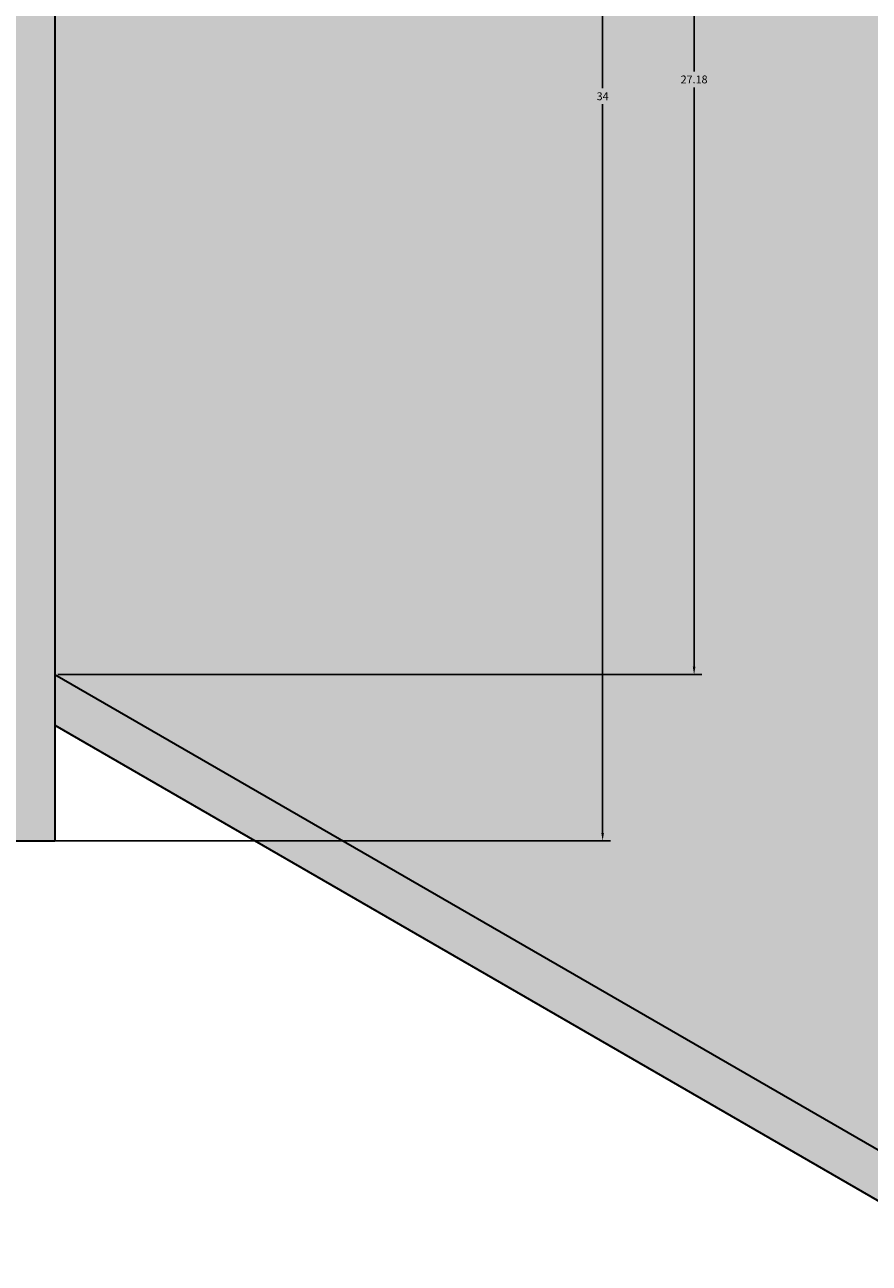
# Model space of a CAD drawing. Units: inches. Extents: x -1 to 292, y -3 to 199.
# Tile 7 of 52: x 23 to 43, y 45 to 73. Entities that reach past the tile are written whole.
import ezdxf

# ---------------------------------------------------------------- set-up
doc = ezdxf.new("R2010")
doc.units = ezdxf.units.IN
doc.header["$MEASUREMENT"] = 0
for name, color, linetype, lineweight in [('M-DIMS', 2, 'Continuous', 18), ('M-EQPM', 7, 'Continuous', 35), ('M-PATT', 8, 'Continuous', 13)]:
    doc.layers.add(name, color=color, linetype=linetype, lineweight=lineweight)
doc.styles.get("Standard").update_dxf_attribs({"font": 'arial.ttf'})
doc.dimstyles.get("Standard").update_dxf_attribs({"dimtxt": 0.18, "dimasz": 0.18, "dimexe": 0.18, "dimexo": 0.0625, "dimgap": 0.09, "dimtad": 0, "dimtih": 1, "dimtoh": 1, "dimdec": 4, "dimzin": 0, "dimdsep": 46, "dimtxsty": 'Standard', "dimcen": 0.09, "dimadec": 0, "dimazin": 0, "dimtfac": 1, "dimtdec": 4, "dimtofl": 0, "dimtmove": 0, "dimatfit": 3, "dimfxl": 1, "dimtolj": 1, "dimtzin": 0, "dimarcsym": 0})

# ---------------------------------------------------------------- blocks, each defined once
blk = doc.blocks.new('DUCT-FLANGE')
for p in [(2.089, 34), (0, 0)]:
    blk.add_line(p, (2.089, 0))
blk = doc.blocks.new('*D7')
at = {"layer": 'Defpoints', "color": 0, "transparency": 16777216}
for p in [(21.861, 54.582), (205.115, 54.582), (21.861, 39.982)]:
    blk.add_point(p, dxfattribs=at)
at = {"layer": 'M-DIMS', "color": 0, "lineweight": -2, "transparency": 16777216}
for p, q in [((21.861, 54.52), (21.861, 39.802)), ((205.115, 54.52), (205.115, 39.802)), ((22.041, 39.982), (113.033, 39.982)), ((204.935, 39.982), (113.944, 39.982))]:
    blk.add_line(p, q, dxfattribs=at)
at = {"layer": 'M-DIMS', "color": 0, "transparency": 16777216}
for points in [[(22.041, 40.012), (22.041, 39.952), (21.861, 39.982)], [(204.935, 40.012), (204.935, 39.952), (205.115, 39.982)]]:
    blk.add_solid(points, dxfattribs=at)
at = {"layer": 'M-DIMS', "color": 0, "transparency": 16777216, "insert": (113.488, 39.982), "char_height": 0.18, "attachment_point": 5}
blk.add_mtext('\\A1;183.25', dxfattribs=at)
blk = doc.blocks.new('*D8')
at = {"layer": 'Defpoints', "color": 0, "transparency": 16777216}
for p in [(-0.662, 126.765), (111.488, 126.765), (69.013, 25.514)]:
    blk.add_point(p, dxfattribs=at)
at = {"layer": 'M-DIMS', "color": 0, "lineweight": -2, "transparency": 16777216}
for p, q in [((111.426, 126.765), (-0.842, 126.765)), ((-0.662, 126.585), (-0.662, 76.321)), ((-0.662, 25.694), (-0.662, 75.958)), ((68.951, 25.514), (-0.842, 25.514))]:
    blk.add_line(p, q, dxfattribs=at)
at = {"layer": 'M-DIMS', "color": 0, "transparency": 16777216}
for points in [[(-0.692, 126.585), (-0.632, 126.585), (-0.662, 126.765)], [(-0.692, 25.694), (-0.632, 25.694), (-0.662, 25.514)]]:
    blk.add_solid(points, dxfattribs=at)
at = {"layer": 'M-DIMS', "color": 0, "transparency": 16777216, "insert": (-0.662, 76.14), "char_height": 0.18, "attachment_point": 5}
blk.add_mtext('\\A1;101.25', dxfattribs=at)
blk = doc.blocks.new('*D14')
at = {"layer": 'Defpoints', "color": 0, "transparency": 16777216}
for p in [(21.861, 88.582), (21.861, 54.582), (36.461, 54.582)]:
    blk.add_point(p, dxfattribs=at)
at = {"layer": 'M-DIMS', "color": 0, "lineweight": -2, "transparency": 16777216}
for p, q in [((21.924, 88.582), (36.641, 88.582)), ((36.461, 88.402), (36.461, 71.764)), ((36.461, 54.762), (36.461, 71.4)), ((21.924, 54.582), (36.641, 54.582))]:
    blk.add_line(p, q, dxfattribs=at)
at = {"layer": 'M-DIMS', "color": 0, "transparency": 16777216}
for points in [[(36.431, 88.402), (36.491, 88.402), (36.461, 88.582)], [(36.431, 54.762), (36.491, 54.762), (36.461, 54.582)]]:
    blk.add_solid(points, dxfattribs=at)
at = {"layer": 'M-DIMS', "color": 0, "transparency": 16777216, "insert": (36.461, 71.582), "char_height": 0.18, "attachment_point": 5}
blk.add_mtext('\\A1;34', dxfattribs=at)
blk = doc.blocks.new('*D17')
at = {"layer": 'Defpoints', "color": 0, "transparency": 16777216}
for p in [(23.95, 85.555), (23.95, 58.376), (38.55, 58.376)]:
    blk.add_point(p, dxfattribs=at)
at = {"layer": 'M-DIMS', "color": 0, "lineweight": -2, "transparency": 16777216}
for p, q in [((24.013, 85.555), (38.73, 85.555)), ((38.55, 85.375), (38.55, 72.147)), ((38.55, 58.556), (38.55, 71.784)), ((24.013, 58.376), (38.73, 58.376))]:
    blk.add_line(p, q, dxfattribs=at)
at = {"layer": 'M-DIMS', "color": 0, "transparency": 16777216}
for points in [[(38.52, 85.375), (38.58, 85.375), (38.55, 85.555)], [(38.52, 58.556), (38.58, 58.556), (38.55, 58.376)]]:
    blk.add_solid(points, dxfattribs=at)
at = {"layer": 'M-DIMS', "color": 0, "transparency": 16777216, "insert": (38.55, 71.966), "char_height": 0.18, "attachment_point": 5}
blk.add_mtext('\\A1;27.18', dxfattribs=at)
blk = doc.blocks.new('*D23')
at = {"layer": 'Defpoints', "color": 0, "transparency": 16777216}
for p in [(21.861, 54.582), (64.679, 51.267), (64.679, -2.71)]:
    blk.add_point(p, dxfattribs=at)
at = {"layer": 'M-DIMS', "color": 0, "lineweight": -2, "transparency": 16777216}
for p, q in [((21.861, 54.52), (21.861, -2.89)), ((64.679, 51.205), (64.679, -2.89)), ((22.041, -2.71), (42.874, -2.71)), ((64.499, -2.71), (43.666, -2.71))]:
    blk.add_line(p, q, dxfattribs=at)
at = {"layer": 'M-DIMS', "color": 0, "transparency": 16777216}
for points in [[(22.041, -2.68), (22.041, -2.74), (21.861, -2.71)], [(64.499, -2.68), (64.499, -2.74), (64.679, -2.71)]]:
    blk.add_solid(points, dxfattribs=at)
at = {"layer": 'M-DIMS', "color": 0, "transparency": 16777216, "insert": (43.27, -2.71), "char_height": 0.18, "attachment_point": 5}
blk.add_mtext('\\A1;42.82', dxfattribs=at)

msp = doc.modelspace()

# ---------------------------------------------------------------- hatches: boundary and pattern name
at = {"layer": 'M-PATT'}
h = msp.add_hatch(color=256, dxfattribs=at)
h.set_gradient(color1=(237, 31, 36), color2=(242, 113, 114), tint=1, name='CYLINDER')
h.paths.add_polyline_path([(106.0735, 105.9941), (106.0735, 106.9941), (108.0603, 106.9941), (107.8488, 107.6501), (57.8007, 107.6501, 0.4142136), (49.9241, 99.7735), (52.3176, 101.3278), (55.0097, 99.7735), (57.4032, 101.3278), (60.0953, 99.7735), (62.4888, 101.3278), (65.1809, 99.7735), (67.5744, 101.3278), (70.2665, 99.7735), (72.66, 101.3278), (75.3521, 99.7735), (77.7456, 101.3278), (80.4377, 99.7735), (82.8312, 101.3278), (85.5233, 99.7735), (87.9168, 101.3278), (90.6089, 99.7735), (93.0024, 101.3278), (95.6945, 99.7735), (98.088, 101.3278), (100.7801, 99.7735), (103.1736, 101.3278), (105.8657, 99.7735), (108.2592, 101.3278), (110.9513, 99.7735), (113.3448, 101.3278), (116.0369, 99.7735), (118.4304, 101.3278), (121.1225, 99.7735), (123.516, 101.3278), (126.2082, 99.7735), (128.6016, 101.3278), (131.2938, 99.7735), (133.6872, 101.3278), (136.3794, 99.7735), (138.7728, 101.3278), (141.465, 99.7735), (143.8584, 101.3278), (146.5506, 99.7735), (148.944, 101.3278), (151.6362, 99.7735), (154.0296, 101.3278), (156.7218, 99.7735), (159.1152, 101.3278), (160.6222, 100.4578), (160.6222, 107.6501), (115.4883, 107.6501), (115.4883, 106.9941), (120.9032, 106.9941), (120.9032, 105.9941), (120.9032, 103.3981), (106.0735, 103.3981)])
h.paths.add_polyline_path([(169.176, 107.6501), (162.1623, 107.6501), (162.1623, 100.004), (164.2008, 101.3278), (166.893, 99.7735), (169.2864, 101.3278), (171.9786, 99.7735), (174.372, 101.3278), (177.0526, 99.7802, 0.4139642)])
h.paths.add_polyline_path([(111.4883, 107.6501), (107.8488, 107.6501), (108.0603, 106.9941), (111.4883, 106.9941)], flags=17)
h.paths.add_polyline_path([(61.6788, 91.897), (57.8007, 91.897, -0.1099266), (54.4604, 92.6403), (43.2011, 92.6403), (23.9502, 84.4688), (23.9502, 58.376), (43.2011, 47.2615), (50.9409, 47.2615, -0.2705926), (57.8007, 51.2672), (61.6788, 51.2672)])
h.paths.add_polyline_path([(73.6788, 91.897), (70.6788, 91.897), (70.6788, 51.2672), (73.6788, 51.2672)])
h.paths.add_polyline_path([(79.6788, 91.897), (76.6788, 91.897), (76.6788, 51.2672), (79.6788, 51.2672)])
h.paths.add_polyline_path([(67.6788, 91.897), (64.6788, 91.897), (64.6788, 51.2672), (67.6788, 51.2672)])
h.paths.add_polyline_path([(101.6788, 91.897), (82.6788, 91.897), (82.6788, 51.2672), (101.6788, 51.2672)])
h.paths.add_polyline_path([(107.6788, 91.897), (104.6788, 91.897), (104.6788, 51.2672), (107.6788, 51.2672)])
h.paths.add_polyline_path([(113.6788, 91.897), (110.6788, 91.897), (110.6788, 51.2672), (113.6788, 51.2672)])
h.paths.add_polyline_path([(119.6788, 91.897), (116.6788, 91.897), (116.6788, 51.2672), (119.6788, 51.2672)])
h.paths.add_polyline_path([(141.6788, 91.897), (122.6788, 91.897), (122.6788, 51.2672), (141.6788, 51.2672)])
h.paths.add_polyline_path([(147.6788, 91.897), (144.6788, 91.897), (144.6788, 51.2672), (147.6788, 51.2672)])
h.paths.add_polyline_path([(153.6788, 91.897), (150.6788, 91.897), (150.6788, 51.2672), (153.6788, 51.2672)])
h.paths.add_polyline_path([(159.6788, 91.897), (156.6788, 91.897), (156.6788, 51.2672), (159.6788, 51.2672)])
h.paths.add_polyline_path([(179.5897, 92.6403), (172.5163, 92.6403, -0.1099266), (169.176, 91.897), (162.6788, 91.897), (162.6788, 51.2672), (169.176, 51.2672, -0.2705926), (176.0358, 47.2615), (179.5897, 47.2615)])
h.paths.add_polyline_path([(203.0265, 84.4688), (183.7755, 92.6403), (181.5897, 92.6403), (181.5897, 47.2615), (183.7755, 47.2615), (203.0265, 58.376)])
h.paths.add_polyline_path([(184.4188, 61.52), (200.7224, 61.52), (200.7224, 77.7532), (184.4188, 77.7532)], flags=24)
h = msp.add_hatch(color=256, dxfattribs=at)
h.set_gradient(color1=(76, 38, 47), color2=(76, 38, 47), tint=1, name='CYLINDER')
h.paths.add_polyline_path([(40.8628, 91.6478), (40.3591, 92.5203), (23.9502, 85.5552), (23.9502, 84.4688)])
h.paths.add_polyline_path([(52.8586, 93.6403), (42.9977, 93.6403), (40.3591, 92.5203), (40.8628, 91.6478), (43.2011, 92.6403), (54.4604, 92.6403, -0.0601508)])
h.paths.add_polyline_path([(23.9502, 88.5821), (21.8612, 88.5821), (21.8612, 54.5821), (23.9502, 54.5821)])
h.paths.add_polyline_path([(23.9502, 58.376), (23.9502, 57.2213), (42.9332, 46.2615), (50.4659, 46.2615, -0.0351813), (50.9409, 47.2615), (43.2011, 47.2615)])
h.paths.add_polyline_path([(179.5897, 93.6403), (174.1181, 93.6403, -0.0601508), (172.5163, 92.6403), (179.5897, 92.6403)])
h.paths.add_polyline_path([(183.979, 93.6403), (181.5897, 93.6403), (181.5897, 92.6403), (183.7755, 92.6403), (203.0265, 84.4688), (203.0265, 85.5552)])
h.paths.add_polyline_path([(205.1155, 88.5821), (203.0265, 88.5821), (203.0265, 54.5821), (205.1155, 54.5821)])
h.paths.add_polyline_path([(203.0265, 57.2213), (203.0265, 58.376), (183.7755, 47.2615), (181.5897, 47.2615), (181.5897, 46.2615), (184.0435, 46.2615)])
h.paths.add_polyline_path([(179.5897, 47.2615), (176.0358, 47.2615, -0.0351813), (176.5107, 46.2615), (179.5897, 46.2615)])

# ---------------------------------------------------------------- linework, layer by layer
at = {"layer": 'M-EQPM'}
for points in [[(23.9502, 58.376), (43.2011, 47.2615), (50.9409, 47.2615)], [(23.9502, 57.2213), (42.9332, 46.2615), (50.4659, 46.2615)]]:
    msp.add_lwpolyline(points, dxfattribs=at)

# ---------------------------------------------------------------- block references
msp.add_blockref('DUCT-FLANGE', (21.861, 54.582), dxfattribs=at)

# ---------------------------------------------------------------- dimensions: what is measured, and where the dimension line sits
at = {"layer": 'M-DIMS'}
for base, p1, p2, angle, override, picture, middle in [((-0.6625, 126.765), (69.013, 25.5141), (111.4883, 126.765), 90, {"dimdec": 2, "dimlfac": 1, "dimrnd": 0, "dimzin": 0, "dimdsep": 46, "dimlunit": 2}, '*D8', (-0.6625, 76.1396)), ((36.4612, 54.5821), (21.8612, 88.5821), (21.8612, 54.5821), 270, {"dimdec": 0, "dimlfac": 1, "dimrnd": 0, "dimzin": 0, "dimdsep": 46, "dimlunit": 2}, '*D14', (36.4612, 71.5821)), ((38.5502, 58.376), (23.9502, 85.5552), (23.9502, 58.376), 270, {"dimdec": 2, "dimlfac": 1, "dimrnd": 0, "dimzin": 0, "dimdsep": 46, "dimlunit": 2}, '*D17', (38.5502, 71.9656)), ((21.8612, 39.9821), (205.1155, 54.5821), (21.8612, 54.5821), 180, {"dimdec": 2, "dimlfac": 1, "dimrnd": 0, "dimzin": 0, "dimdsep": 46, "dimlunit": 2}, '*D7', (113.4883, 39.9821))]:
    dim = msp.add_linear_dim(base=base, p1=p1, p2=p2, angle=angle, dimstyle='Standard', override=override, dxfattribs=at)
    dim.commit()
    dim.dimension.update_dxf_attribs({"geometry": picture, "text_midpoint": middle})
dim = msp.add_linear_dim(base=(64.6788, -2.7104), p1=(21.8612, 54.5821), p2=(64.6788, 51.2672), dimstyle='Standard', override={"dimdec": 2, "dimlfac": 1, "dimrnd": 0, "dimzin": 0, "dimdsep": 46, "dimlunit": 2}, dxfattribs=at)
dim.commit()
dim.dimension.update_dxf_attribs({"geometry": '*D23', "text_midpoint": (43.27, -2.7104)})

doc.saveas('drawing.dxf')
